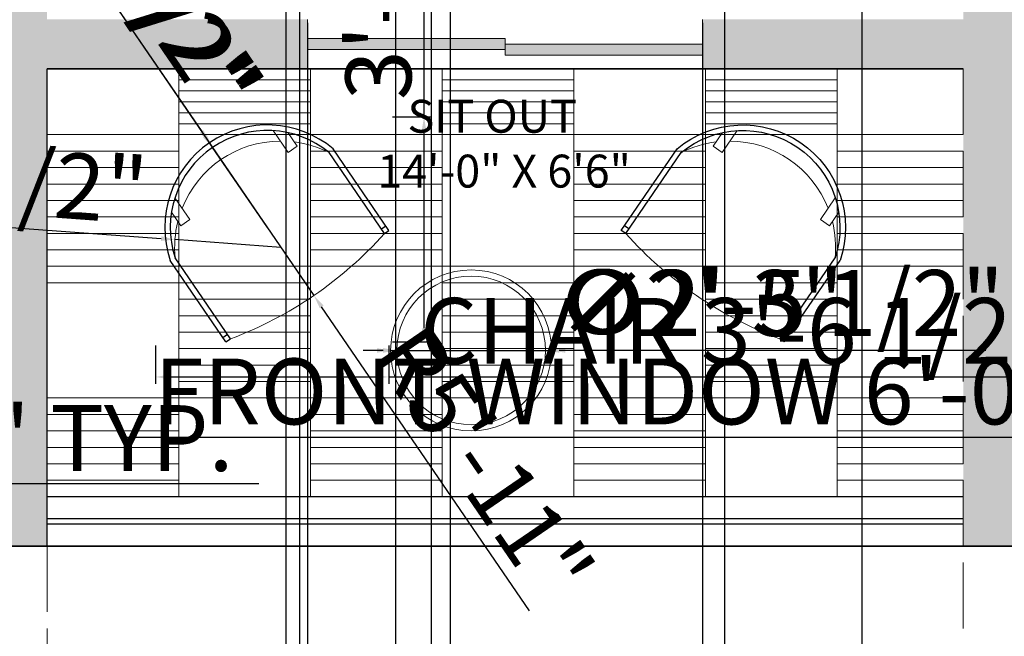
# Model space of a CAD drawing. Units: millimetres. Extents: x 542930 to 543750, y 628093 to 628738.
# Tile 5 of 14: x 543153 to 543333, y 628237 to 628350. Entities that reach past the tile are written whole.
import ezdxf

# ---------------------------------------------------------------- set-up
doc = ezdxf.new("R2010")
doc.units = ezdxf.units.MM
doc.linetypes.add('ACAD_ISO02W100', pattern=[15, 12, -3])
for name, color, linetype, lineweight in [('A-ANNO-DIMS', 2, 'Continuous', 18), ('A-FLOR-BELO', 4, 'ACAD_ISO02W100', 18), ('A-FLOR-EDGE', 9, 'Continuous', 25), ('A-FURN', 8, 'Continuous', 18), ('A-WALL', 7, 'Continuous', 35), ('DOORS', 30, 'Continuous', 18)]:
    doc.layers.add(name, color=color, linetype=linetype, lineweight=lineweight)
for name, color, linetype, lineweight, true_color in [('A-AREA-IDEN', 40, 'Continuous', 18, 0xf8d731), ('A-DOOR-PATT', 152, 'Continuous', 13, 0x2776bb), ('A-FLOR-DECK-PATT', 32, 'Continuous', 13, 0xcd6928), ('A-WALL-PATT', 251, 'Continuous', 13, 0x636466)]:
    doc.layers.add(name, color=color, linetype=linetype, lineweight=lineweight, true_color=true_color)
doc.layers.add('TEXT', color=220, linetype='Continuous')
doc.styles.get("Standard").update_dxf_attribs({"font": 'arial.ttf'})
doc.dimstyles.new('ISO-25', dxfattribs={"dimtxt": 12, "dimasz": 2.5, "dimexe": 1.25, "dimexo": 0.625, "dimtad": 1, "dimdec": 0, "dimlunit": 3, "dimtxsty": 'Standard', "dimcen": 2.5, "dimadec": 0, "dimazin": 0, "dimtfac": 1, "dimtdec": 0, "dimtmove": 0, "dimatfit": 3, "dimfxl": 1, "dimarcsym": 0})

# ---------------------------------------------------------------- blocks, each defined once
blk = doc.blocks.new('chair')
for p, q in [((543076.08, 628228.18), (543073.37, 628232.15)), ((543076.04, 628231.79), (543077.73, 628229.31)), ((543077.73, 628229.31), (543076.08, 628228.18)), ((543058.18, 628215.93), (543055.46, 628219.91)), ((543054.84, 628217.28), (543056.53, 628214.81)), ((543056.53, 628214.81), (543058.18, 628215.93))]:
    blk.add_line(p, q)
for centre, radius, start, end in [((543074.79, 628210.87), 19.38, 90.3414, 158.4163), ((543074.79, 628210.87), 19.38, 63.0526, 82.8533), ((543074.79, 628210.87), 19.38, 165.9044, 185.7051), ((543040.66, 628260.76), 71.07, 290.5394, 318.2183)]:
    blk.add_arc(centre, radius, start, end)
at = {"layer": 'TEXT'}
for p, q in [((543093.65, 628213.4), (543083.57, 628228.14)), ((543094.48, 628213.97), (543084.31, 628228.82)), ((543093.09, 628214.23), (543093.91, 628214.79)), ((543093.65, 628213.4), (543094.48, 628213.97)), ((543064.77, 628193.64), (543054.6, 628208.5)), ((543065.59, 628194.21), (543055.51, 628208.95)), ((543064.2, 628194.47), (543065.03, 628195.03)), ((543064.77, 628193.64), (543065.59, 628194.21))]:
    blk.add_line(p, q, dxfattribs=at)
for radius, start, end in [(18.7, 50.0638, 198.6939), (17.7, 50.5038, 198.2539)]:
    blk.add_arc((543072.31, 628214.49), radius, start, end, dxfattribs=at)
blk = doc.blocks.new('*D41')
at = {"layer": 'A-ANNO-DIMS', "color": 0, "lineweight": -2, "transparency": 16777216}
for p, q in [((543177.94, 628290.42), (543177.94, 628283.41)), ((543220.5, 628290.42), (543220.5, 628283.41)), ((543180.44, 628284.66), (543218, 628284.66)), ((543220.5, 628284.66), (543382.04, 628284.66))]:
    blk.add_line(p, q, dxfattribs=at)
at = {"layer": 'A-ANNO-DIMS', "color": 0, "transparency": 16777216}
for points in [[(543180.44, 628285.08), (543180.44, 628284.25), (543177.94, 628284.66)], [(543218, 628285.08), (543218, 628284.25), (543220.5, 628284.66)]]:
    blk.add_solid(points, dxfattribs=at)
at = {"layer": 'Defpoints', "color": 0, "transparency": 16777216}
for p in [(543177.94, 628291.05), (543220.5, 628291.05), (543220.5, 628284.66)]:
    blk.add_point(p, dxfattribs=at)
at = {"layer": 'A-ANNO-DIMS', "color": 0, "transparency": 16777216, "insert": (543302.52, 628291.5), "char_height": 12, "attachment_point": 5}
blk.add_mtext('CHAIR 3\'-6 1/2" TYP.', dxfattribs=at)
blk = doc.blocks.new('*D42')
at = {"layer": 'A-ANNO-DIMS', "color": 0, "lineweight": -2, "transparency": 16777216}
for p, q in [((543226.89, 628332.06), (543226.89, 628408.95)), ((543221.13, 628332.06), (543228.14, 628332.06)), ((543226.89, 628293.55), (543226.89, 628329.56)), ((543221.13, 628291.05), (543228.14, 628291.05))]:
    blk.add_line(p, q, dxfattribs=at)
at = {"layer": 'A-ANNO-DIMS', "color": 0, "transparency": 16777216}
for points in [[(543226.47, 628329.56), (543227.3, 628329.56), (543226.89, 628332.06)], [(543226.47, 628293.55), (543227.3, 628293.55), (543226.89, 628291.05)]]:
    blk.add_solid(points, dxfattribs=at)
at = {"layer": 'Defpoints', "color": 0, "transparency": 16777216}
for p in [(543220.5, 628332.06), (543226.89, 628332.06), (543220.5, 628291.05)]:
    blk.add_point(p, dxfattribs=at)
at = {"layer": 'A-ANNO-DIMS', "color": 0, "transparency": 16777216, "insert": (543220.13, 628371.75), "char_height": 12, "attachment_point": 5, "rotation": 90}
blk.add_mtext('3\'-5" TYP.', dxfattribs=at)
blk = doc.blocks.new('*D47')
at = {"layer": 'A-ANNO-DIMS', "color": 0, "lineweight": -2, "transparency": 16777216}
for p, q in [((542998.67, 628268.2), (542998.67, 628263.97)), ((543022.69, 628268.2), (543022.69, 628263.97)), ((543001.17, 628265.22), (543020.19, 628265.22)), ((543022.69, 628265.22), (543196.77, 628265.22))]:
    blk.add_line(p, q, dxfattribs=at)
at = {"layer": 'A-ANNO-DIMS', "color": 0, "transparency": 16777216}
for points in [[(543001.17, 628265.64), (543001.17, 628264.81), (542998.67, 628265.22)], [(543020.19, 628265.64), (543020.19, 628264.81), (543022.69, 628265.22)]]:
    blk.add_solid(points, dxfattribs=at)
at = {"layer": 'Defpoints', "color": 0, "transparency": 16777216}
for p in [(542998.67, 628268.83), (543022.69, 628268.83), (543022.69, 628265.22)]:
    blk.add_point(p, dxfattribs=at)
at = {"layer": 'A-ANNO-DIMS', "color": 0, "transparency": 16777216, "insert": (543110.98, 628271.97), "char_height": 12, "attachment_point": 5}
blk.add_mtext('END TABLE 2\'-0" TYP.', dxfattribs=at)
blk = doc.blocks.new('*D49')
at = {"layer": 'A-ANNO-DIMS', "color": 0, "lineweight": -2, "transparency": 16777216}
for p, q in [((543388.65, 628263.45), (543388.65, 628274.88)), ((543460.65, 628263.45), (543460.65, 628274.88)), ((543388.65, 628273.63), (543171.83, 628273.63)), ((543458.15, 628273.63), (543391.15, 628273.63))]:
    blk.add_line(p, q, dxfattribs=at)
at = {"layer": 'A-ANNO-DIMS', "color": 0, "transparency": 16777216}
for points in [[(543391.15, 628274.04), (543391.15, 628273.21), (543388.65, 628273.63)], [(543458.15, 628274.04), (543458.15, 628273.21), (543460.65, 628273.63)]]:
    blk.add_solid(points, dxfattribs=at)
at = {"layer": 'Defpoints', "color": 0, "transparency": 16777216}
for p in [(543388.65, 628273.63), (543388.65, 628262.83), (543460.65, 628262.83)]:
    blk.add_point(p, dxfattribs=at)
at = {"layer": 'A-ANNO-DIMS', "color": 0, "transparency": 16777216, "insert": (543278.99, 628280.46), "char_height": 12, "attachment_point": 5}
blk.add_mtext('FRONT WINDOW 6\'-0" TYP.', dxfattribs=at)
blk = doc.blocks.new('*D61')
at = {"layer": 'A-ANNO-DIMS', "color": 0, "lineweight": -2, "transparency": 16777216}
for p, q in [((543500.29, 628253.83), (543537.81, 628253.83)), ((543536.56, 628136.33), (543536.56, 628251.33)), ((543325.79, 628133.83), (543537.81, 628133.83))]:
    blk.add_line(p, q, dxfattribs=at)
at = {"layer": 'A-ANNO-DIMS', "color": 0, "transparency": 16777216}
for points in [[(543536.15, 628251.33), (543536.98, 628251.33), (543536.56, 628253.83)], [(543536.15, 628136.33), (543536.98, 628136.33), (543536.56, 628133.83)]]:
    blk.add_solid(points, dxfattribs=at)
at = {"layer": 'Defpoints', "color": 0, "transparency": 16777216}
for p in [(543499.67, 628253.83), (543536.56, 628253.83), (543325.17, 628133.83)]:
    blk.add_point(p, dxfattribs=at)
at = {"layer": 'A-ANNO-DIMS', "color": 0, "transparency": 16777216, "insert": (543529.81, 628193.83), "char_height": 12, "attachment_point": 5, "rotation": 90}
blk.add_mtext('10\'-0"', dxfattribs=at)
blk = doc.blocks.new('*D71')
at = {"layer": 'A-ANNO-DIMS', "color": 0, "lineweight": -2, "transparency": 16777216}
for p, q in [((543201.67, 628544.2), (543201.67, 628103.84)), ((543281.67, 628544.2), (543281.67, 628103.84)), ((543204.17, 628105.09), (543279.17, 628105.09))]:
    blk.add_line(p, q, dxfattribs=at)
at = {"layer": 'A-ANNO-DIMS', "color": 0, "transparency": 16777216}
for points in [[(543204.17, 628105.5), (543204.17, 628104.67), (543201.67, 628105.09)], [(543279.17, 628105.5), (543279.17, 628104.67), (543281.67, 628105.09)]]:
    blk.add_solid(points, dxfattribs=at)
at = {"layer": 'Defpoints', "color": 0, "transparency": 16777216}
for p in [(543201.67, 628544.83), (543281.67, 628544.83), (543281.67, 628105.09)]:
    blk.add_point(p, dxfattribs=at)
at = {"layer": 'A-ANNO-DIMS', "color": 0, "transparency": 16777216, "insert": (543241.67, 628111.84), "char_height": 12, "attachment_point": 5}
blk.add_mtext('6\'-8"', dxfattribs=at)
blk = doc.blocks.new('*D76')
at = {"layer": 'A-ANNO-DIMS', "color": 0, "lineweight": -2, "transparency": 16777216}
for p, q in [((543205.67, 628349.2), (543205.67, 628103.84)), ((543277.67, 628349.2), (543277.67, 628103.84)), ((543208.17, 628105.09), (543275.17, 628105.09))]:
    blk.add_line(p, q, dxfattribs=at)
at = {"layer": 'A-ANNO-DIMS', "color": 0, "transparency": 16777216}
for points in [[(543208.17, 628105.5), (543208.17, 628104.67), (543205.67, 628105.09)], [(543275.17, 628105.5), (543275.17, 628104.67), (543277.67, 628105.09)]]:
    blk.add_solid(points, dxfattribs=at)
at = {"layer": 'Defpoints', "color": 0, "transparency": 16777216}
for p in [(543205.67, 628349.83), (543277.67, 628349.83), (543277.67, 628105.09)]:
    blk.add_point(p, dxfattribs=at)
at = {"layer": 'A-ANNO-DIMS', "color": 0, "transparency": 16777216, "insert": (543241.67, 628111.84), "char_height": 12, "attachment_point": 5}
blk.add_mtext('6\'-0"', dxfattribs=at)
blk = doc.blocks.new('*D79')
at = {"layer": 'A-ANNO-DIMS', "color": 0, "lineweight": -2, "transparency": 16777216}
for p, q in [((543204.19, 628433.96), (543204.19, 628103.84)), ((543228.16, 628433.96), (543228.16, 628103.84)), ((543206.69, 628105.09), (543225.66, 628105.09)), ((543228.16, 628105.09), (543264.02, 628105.09))]:
    blk.add_line(p, q, dxfattribs=at)
at = {"layer": 'A-ANNO-DIMS', "color": 0, "transparency": 16777216}
for points in [[(543206.69, 628105.5), (543206.69, 628104.67), (543204.19, 628105.09)], [(543225.66, 628105.5), (543225.66, 628104.67), (543228.16, 628105.09)]]:
    blk.add_solid(points, dxfattribs=at)
at = {"layer": 'Defpoints', "color": 0, "transparency": 16777216}
for p in [(543204.19, 628434.59), (543228.16, 628434.59), (543228.16, 628105.09)]:
    blk.add_point(p, dxfattribs=at)
at = {"layer": 'A-ANNO-DIMS', "color": 0, "transparency": 16777216, "insert": (543247.34, 628111.84), "char_height": 12, "attachment_point": 5}
blk.add_mtext('2\'-0"', dxfattribs=at)
blk = doc.blocks.new('*D81')
at = {"layer": 'A-ANNO-DIMS', "color": 0, "lineweight": -2, "transparency": 16777216}
for p, q in [((543228.16, 628433.96), (543228.16, 628103.84)), ((543306.67, 628434.2), (543306.67, 628103.84)), ((543230.66, 628105.09), (543304.17, 628105.09))]:
    blk.add_line(p, q, dxfattribs=at)
at = {"layer": 'A-ANNO-DIMS', "color": 0, "transparency": 16777216}
for points in [[(543230.66, 628105.5), (543230.66, 628104.67), (543228.16, 628105.09)], [(543304.17, 628105.5), (543304.17, 628104.67), (543306.67, 628105.09)]]:
    blk.add_solid(points, dxfattribs=at)
at = {"layer": 'Defpoints', "color": 0, "transparency": 16777216}
for p in [(543228.16, 628434.59), (543306.67, 628434.83), (543306.67, 628105.09)]:
    blk.add_point(p, dxfattribs=at)
at = {"layer": 'A-ANNO-DIMS', "color": 0, "transparency": 16777216, "insert": (543267.41, 628111.92), "char_height": 12, "attachment_point": 5}
blk.add_mtext('6\'-6 1/2"', dxfattribs=at)
blk = doc.blocks.new('*D87')
at = {"layer": 'A-ANNO-DIMS', "color": 0, "lineweight": -2, "transparency": 16777216}
for p, q in [((543221.67, 628580.2), (543221.67, 628103.84)), ((543231.67, 628580.2), (543231.67, 628103.84)), ((543224.17, 628105.09), (543229.17, 628105.09)), ((543231.67, 628105.09), (543276.64, 628105.09))]:
    blk.add_line(p, q, dxfattribs=at)
at = {"layer": 'A-ANNO-DIMS', "color": 0, "transparency": 16777216}
for points in [[(543224.17, 628105.5), (543224.17, 628104.67), (543221.67, 628105.09)], [(543229.17, 628105.5), (543229.17, 628104.67), (543231.67, 628105.09)]]:
    blk.add_solid(points, dxfattribs=at)
at = {"layer": 'Defpoints', "color": 0, "transparency": 16777216}
for p in [(543221.67, 628580.83), (543231.67, 628580.83), (543231.67, 628105.09)]:
    blk.add_point(p, dxfattribs=at)
at = {"layer": 'A-ANNO-DIMS', "color": 0, "transparency": 16777216, "insert": (543255.4, 628111.84), "char_height": 12, "attachment_point": 5}
blk.add_mtext('0\'-10"', dxfattribs=at)
blk = doc.blocks.new('*D88')
at = {"layer": 'A-ANNO-DIMS', "color": 0, "lineweight": -2, "transparency": 16777216}
for p, q in [((543218.3, 628289.5), (543215.8, 628289.5)), ((543220.8, 628289.5), (543250.15, 628289.5)), ((543329.31, 628289.5), (543252.65, 628289.5))]:
    blk.add_line(p, q, dxfattribs=at)
at = {"layer": 'A-ANNO-DIMS', "color": 0, "transparency": 16777216}
for points in [[(543218.3, 628289.91), (543218.3, 628289.08), (543220.8, 628289.5)], [(543252.65, 628289.91), (543252.65, 628289.08), (543250.15, 628289.5)]]:
    blk.add_solid(points, dxfattribs=at)
at = {"layer": 'Defpoints', "color": 0, "transparency": 16777216}
for p in [(543220.8, 628289.5), (543250.15, 628289.5)]:
    blk.add_point(p, dxfattribs=at)
at = {"layer": 'A-ANNO-DIMS', "color": 0, "transparency": 16777216, "insert": (543292.23, 628296.59), "char_height": 12, "attachment_point": 5, "rotation": 0.0001}
blk.add_mtext('∅2\'-5 1/2"', dxfattribs=at)
blk = doc.blocks.new('*D89')
at = {"layer": 'A-ANNO-DIMS', "color": 0, "lineweight": -2, "transparency": 16777216}
for p, q in [((543219.43, 628289.5), (543216.93, 628289.5)), ((543221.93, 628289.5), (543249.02, 628289.5)), ((543300.22, 628289.5), (543251.52, 628289.5))]:
    blk.add_line(p, q, dxfattribs=at)
at = {"layer": 'A-ANNO-DIMS', "color": 0, "transparency": 16777216}
for points in [[(543219.43, 628289.91), (543219.43, 628289.08), (543221.93, 628289.5)], [(543251.52, 628289.91), (543251.52, 628289.08), (543249.02, 628289.5)]]:
    blk.add_solid(points, dxfattribs=at)
at = {"layer": 'Defpoints', "color": 0, "transparency": 16777216}
for p in [(543221.93, 628289.5), (543249.02, 628289.5)]:
    blk.add_point(p, dxfattribs=at)
at = {"layer": 'A-ANNO-DIMS', "color": 0, "transparency": 16777216, "insert": (543277.12, 628296.59), "char_height": 12, "attachment_point": 5, "rotation": 0.0001}
blk.add_mtext('∅2\'-3"', dxfattribs=at)
blk = doc.blocks.new('*D92')
at = {"layer": 'A-ANNO-DIMS', "color": 0, "lineweight": -2, "transparency": 16777216}
for p, q in [((543166.68, 628358.16), (543206.81, 628299.51)), ((543246.12, 628242.05), (543208.22, 628297.45))]:
    blk.add_line(p, q, dxfattribs=at)
at = {"layer": 'A-ANNO-DIMS', "color": 0, "transparency": 16777216}
blk.add_solid([(543208.57, 628297.68), (543207.88, 628297.21), (543206.81, 628299.51)], dxfattribs=at)
at = {"layer": 'Defpoints', "color": 0, "transparency": 16777216}
for p in [(543166.68, 628358.16), (543206.81, 628299.51)]:
    blk.add_point(p, dxfattribs=at)
at = {"layer": 'A-ANNO-DIMS', "color": 0, "transparency": 16777216, "insert": (543236.46, 628268.13), "char_height": 12, "attachment_point": 5, "rotation": 304.379}
blk.add_mtext('R5\'-11"', dxfattribs=at)
blk = doc.blocks.new('*D93')
at = {"layer": 'A-ANNO-DIMS', "color": 0, "lineweight": -2, "transparency": 16777216}
for p, q in [((543078.39, 628317.26), (543178.99, 628309.88)), ((543200.81, 628308.28), (543181.49, 628309.7))]:
    blk.add_line(p, q, dxfattribs=at)
at = {"layer": 'A-ANNO-DIMS', "color": 0, "transparency": 16777216}
blk.add_solid([(543179.02, 628310.3), (543178.96, 628309.46), (543181.49, 628309.7)], dxfattribs=at)
at = {"layer": 'Defpoints', "color": 0, "transparency": 16777216}
for p in [(543181.49, 628309.7), (543200.81, 628308.28)]:
    blk.add_point(p, dxfattribs=at)
at = {"layer": 'A-ANNO-DIMS', "color": 0, "transparency": 16777216, "insert": (543127.94, 628320.48), "char_height": 12, "attachment_point": 5, "rotation": 355.8053}
blk.add_mtext('3X R1\'-7 1/2"', dxfattribs=at)
blk = doc.blocks.new('*D94')
at = {"layer": 'A-ANNO-DIMS', "color": 0, "lineweight": -2, "transparency": 16777216}
for p, q in [((543143.96, 628391.37), (543186.37, 628329.39)), ((543198.34, 628311.9), (543187.78, 628327.33))]:
    blk.add_line(p, q, dxfattribs=at)
at = {"layer": 'A-ANNO-DIMS', "color": 0, "transparency": 16777216}
blk.add_solid([(543186.71, 628329.63), (543186.02, 628329.15), (543187.78, 628327.33)], dxfattribs=at)
at = {"layer": 'Defpoints', "color": 0, "transparency": 16777216}
for p in [(543187.78, 628327.33), (543198.34, 628311.9)]:
    blk.add_point(p, dxfattribs=at)
at = {"layer": 'A-ANNO-DIMS', "color": 0, "transparency": 16777216, "insert": (543170.1, 628365.27), "char_height": 12, "attachment_point": 5, "rotation": 304.3793}
blk.add_mtext('R1\'-6 1/2"', dxfattribs=at)
blk = doc.blocks.new('*D95')
at = {"layer": 'A-ANNO-DIMS', "color": 0, "lineweight": -2, "transparency": 16777216}
for p, q in [((543144.53, 628390.54), (543186.93, 628328.57)), ((543198.34, 628311.9), (543188.34, 628326.5))]:
    blk.add_line(p, q, dxfattribs=at)
at = {"layer": 'A-ANNO-DIMS', "color": 0, "transparency": 16777216}
blk.add_solid([(543187.28, 628328.8), (543186.59, 628328.33), (543188.34, 628326.5)], dxfattribs=at)
at = {"layer": 'Defpoints', "color": 0, "transparency": 16777216}
for p in [(543188.34, 628326.5), (543198.34, 628311.9)]:
    blk.add_point(p, dxfattribs=at)
at = {"layer": 'A-ANNO-DIMS', "color": 0, "transparency": 16777216, "insert": (543170.66, 628364.44), "char_height": 12, "attachment_point": 5, "rotation": 304.3778}
blk.add_mtext('R1\'-5 1/2"', dxfattribs=at)

msp = doc.modelspace()

# ---------------------------------------------------------------- hatches: boundary and pattern name
at = {"layer": 'A-DOOR-PATT'}
h = msp.add_hatch(color=256, dxfattribs=at)
h.dxf.hatch_style = 1
h.paths.add_polyline_path([(543241.67, 628346.33), (543205.67, 628346.33), (543205.67, 628344.33), (543241.67, 628344.33)])
h = msp.add_hatch(color=256, dxfattribs=at)
h.dxf.hatch_style = 1
h.paths.add_polyline_path([(543277.67, 628345.33), (543241.67, 628345.33), (543241.67, 628344.33), (543241.67, 628343.33), (543277.67, 628343.33)])
at = {"layer": 'A-FLOR-DECK-PATT'}
h = msp.add_hatch(dxfattribs=at)
h.set_pattern_fill('LINE', color=256, scale=0.629922088, style=0)
h.paths.add_polyline_path([(543182.17, 628328.88), (543206.17, 628328.88), (543206.17, 628340.77), (543182.17, 628340.77)])
h = msp.add_hatch(dxfattribs=at)
h.set_pattern_fill('LINE', color=256, scale=0.629922088, style=0)
h.paths.add_polyline_path([(543230.17, 628328.88), (543254.17, 628328.88), (543254.17, 628340.77), (543230.17, 628340.77)])
h = msp.add_hatch(dxfattribs=at)
h.set_pattern_fill('LINE', color=256, scale=0.629922088, style=0)
h.paths.add_polyline_path([(543278.17, 628328.88), (543302.17, 628328.88), (543302.17, 628340.77), (543278.17, 628340.77)])
h = msp.add_hatch(dxfattribs=at)
h.set_pattern_fill('LINE', color=256, scale=0.94488163, style=0)
h.paths.add_polyline_path([(543158.17, 628304.88), (543182.17, 628304.88), (543182.17, 628328.77), (543158.17, 628328.77)])
h = msp.add_hatch(dxfattribs=at)
h.set_pattern_fill('LINE', color=256, scale=0.94488163, style=0)
h.paths.add_polyline_path([(543206.17, 628304.88), (543230.17, 628304.88), (543230.17, 628328.77), (543206.17, 628328.77)])
h = msp.add_hatch(dxfattribs=at)
h.set_pattern_fill('LINE', color=256, scale=0.94488163, style=0)
h.paths.add_polyline_path([(543254.17, 628304.88), (543278.17, 628304.88), (543278.17, 628328.77), (543254.17, 628328.77)])
h = msp.add_hatch(dxfattribs=at)
h.set_pattern_fill('LINE', color=256, scale=0.94488163, style=0)
h.paths.add_polyline_path([(543302.17, 628304.88), (543325.17, 628304.88), (543325.17, 628328.77), (543302.17, 628328.77)])
h = msp.add_hatch(dxfattribs=at)
h.set_pattern_fill('LINE', color=256, scale=0.94488163, style=0)
h.paths.add_polyline_path([(543230.17, 628280.88), (543254.17, 628280.88), (543254.17, 628304.77), (543230.17, 628304.77)])
h = msp.add_hatch(dxfattribs=at)
h.set_pattern_fill('LINE', color=256, scale=0.94488163, style=0)
h.paths.add_polyline_path([(543278.17, 628280.88), (543302.17, 628280.88), (543302.17, 628304.77), (543278.17, 628304.77)])
h = msp.add_hatch(dxfattribs=at)
h.set_pattern_fill('LINE', color=256, scale=0.94488163, style=0)
h.paths.add_polyline_path([(543182.17, 628280.88), (543206.17, 628280.88), (543206.17, 628301.77), (543182.17, 628301.77)])
h = msp.add_hatch(dxfattribs=at)
h.set_pattern_fill('LINE', color=256, scale=0.94488163, style=0)
h.paths.add_polyline_path([(543158.17, 628262.88), (543182.17, 628262.88), (543182.17, 628280.77), (543158.17, 628280.77)])
h = msp.add_hatch(dxfattribs=at)
h.set_pattern_fill('LINE', color=256, scale=0.94488163, style=0)
h.paths.add_polyline_path([(543206.17, 628262.88), (543230.17, 628262.88), (543230.17, 628280.77), (543206.17, 628280.77)])
h = msp.add_hatch(dxfattribs=at)
h.set_pattern_fill('LINE', color=256, scale=0.94488163, style=0)
h.paths.add_polyline_path([(543254.17, 628262.88), (543278.17, 628262.88), (543278.17, 628280.77), (543254.17, 628280.77)])
h = msp.add_hatch(dxfattribs=at)
h.set_pattern_fill('LINE', color=256, scale=0.94488163, style=0)
h.paths.add_polyline_path([(543302.17, 628262.88), (543325.17, 628262.88), (543325.17, 628280.77), (543302.17, 628280.77)])
at = {"layer": 'A-WALL-PATT'}
h = msp.add_hatch(color=256, dxfattribs=at)
h.dxf.hatch_style = 1
h.paths.add_polyline_path([(543388.65, 628262.83), (543374.28, 628262.83), (543334.17, 628262.83), (543334.17, 628439.36), (543325.17, 628439.36), (543325.17, 628349.83), (543277.67, 628349.83), (543277.67, 628340.83), (543325.17, 628340.83), (543325.17, 628253.83), (543388.65, 628253.83)])
h = msp.add_hatch(color=256, dxfattribs=at)
h.dxf.hatch_style = 1
h.paths.add_polyline_path([(543158.17, 628340.83), (543205.67, 628340.83), (543205.67, 628349.83), (543158.17, 628349.83), (543158.17, 628360.23), (543149.17, 628360.23), (543149.17, 628262.83), (543094.69, 628262.83), (543094.69, 628253.83), (543158.17, 628253.83)])

# ---------------------------------------------------------------- linework, layer by layer
at = {"layer": 'A-FLOR-BELO'}
for p, q in [((543325.17, 628340.83), (543325.17, 628133.83)), ((543158.17, 628253.83), (543158.17, 628133.79))]:
    msp.add_line(p, q, dxfattribs=at)
at = {"layer": 'A-FLOR-DECK-PATT'}
for p, q in [((543182.17, 628262.83), (543182.17, 628340.83)), ((543206.17, 628262.83), (543206.17, 628340.83)), ((543230.17, 628262.83), (543230.17, 628340.83)), ((543254.17, 628262.83), (543254.17, 628340.83)), ((543278.17, 628262.83), (543278.17, 628340.83)), ((543302.17, 628262.83), (543302.17, 628340.83)), ((543325.17, 628328.83), (543158.17, 628328.83)), ((543325.17, 628304.83), (543158.17, 628304.83)), ((543206.17, 628301.83), (543158.17, 628301.83)), ((543325.17, 628280.83), (543158.17, 628280.83))]:
    msp.add_line(p, q, dxfattribs=at)
at = {"layer": 'A-FLOR-EDGE'}
for p, q in [((543158.17, 628253.83), (543158.17, 628340.83)), ((543325.17, 628262.83), (543158.17, 628262.83)), ((543325.17, 628258.83), (543158.17, 628258.83))]:
    msp.add_line(p, q, dxfattribs=at)
msp.add_lwpolyline([(543325.17, 628257.83), (543158.17, 628257.83)], dxfattribs=at)
at = {"layer": 'A-FURN'}
for radius in [14.67, 13.54]:
    msp.add_circle((543235.47, 628289.5), radius, dxfattribs=at)
at = {"layer": 'A-WALL'}
msp.add_line((543325.17, 628340.83), (543158.17, 628340.83), dxfattribs=at)
msp.add_lwpolyline([(543499.67, 628253.83), (542983.67, 628253.83), (542983.67, 628589.83)], dxfattribs=at)
at = {"layer": 'DOORS'}
for p, q in [((543205.67, 628349.83), (543205.67, 628340.83)), ((543277.67, 628349.83), (543277.67, 628340.83)), ((543205.67, 628346.33), (543241.67, 628346.33)), ((543241.67, 628346.33), (543241.67, 628343.33)), ((543205.67, 628344.33), (543241.67, 628344.33)), ((543241.67, 628345.33), (543277.67, 628345.33)), ((543241.67, 628343.33), (543277.67, 628343.33))]:
    msp.add_line(p, q, dxfattribs=at)

# ---------------------------------------------------------------- block references
at = {"layer": 'A-FURN'}
msp.add_blockref('chair', (126.02, 97.41), dxfattribs=at)
at = {"layer": 'A-FURN', "xscale": -1}
msp.add_blockref('chair', (1086357.31, 97.41), dxfattribs=at)

# ---------------------------------------------------------------- texts
at = {"layer": 'A-AREA-IDEN', "insert": (543216.54, 628335.18), "char_height": 6, "attachment_point": 1}
msp.add_mtext_dynamic_manual_height_columns('    SIT OUT\\P 14\'-0" X 6\'6"', width=77.2525, gutter_width=12.5, heights=[0], dxfattribs=at)

# ---------------------------------------------------------------- dimensions: what is measured, and where the dimension line sits
at = {"layer": 'A-ANNO-DIMS'}
for base, p1, p2, picture, middle in [((543231.67, 628105.09), (543221.67, 628580.83), (543231.67, 628580.83), '*D87', (543255.4, 628111.84)), ((543281.67, 628105.09), (543201.67, 628544.83), (543281.67, 628544.83), '*D71', (543241.67, 628111.84)), ((543228.16, 628105.09), (543204.19, 628434.59), (543228.16, 628434.59), '*D79', (543247.34, 628111.84)), ((543306.67, 628105.09), (543228.16, 628434.59), (543306.67, 628434.83), '*D81', (543267.41, 628111.92)), ((543277.67, 628105.09), (543205.67, 628349.83), (543277.67, 628349.83), '*D76', (543241.67, 628111.84))]:
    dim = msp.add_linear_dim(base=base, p1=p1, p2=p2, dimstyle='ISO-25', override={"dimdec": 1, "dimlfac": 1, "dimrnd": 0, "dimzin": 1, "dimdsep": 46, "dimlunit": 4, "dimfrac": 2}, dxfattribs=at)
    dim.commit()
    dim.dimension.update_dxf_attribs({"geometry": picture, "text_midpoint": middle})
for base, p1, p2, angle, text, picture, middle in [((543226.89, 628332.06), (543220.5, 628291.05), (543220.5, 628332.06), 90, '<> TYP.', '*D42', (543220.13, 628371.75)), ((543388.65, 628273.63), (543460.65, 628262.83), (543388.65, 628262.83), 180, 'FRONT WINDOW <> TYP.', '*D49', (543278.99, 628280.46))]:
    dim = msp.add_linear_dim(base=base, p1=p1, p2=p2, angle=angle, text=text, dimstyle='ISO-25', override={"dimdec": 1, "dimlfac": 1, "dimrnd": 0, "dimzin": 1, "dimdsep": 46, "dimlunit": 4, "dimfrac": 2}, dxfattribs=at)
    dim.commit()
    dim.dimension.update_dxf_attribs({"geometry": picture, "text_midpoint": middle})
for mpoint, picture, middle in [((543187.78, 628327.33), '*D94', (543170.1, 628365.27)), ((543188.34, 628326.5), '*D95', (543170.66, 628364.44))]:
    dim = msp.add_radius_dim(center=(543198.34, 628311.9), mpoint=mpoint, dimstyle='ISO-25', override={"dimdec": 1, "dimlfac": 1, "dimrnd": 0, "dimzin": 1, "dimdsep": 46, "dimlunit": 4, "dimfrac": 2}, dxfattribs=at)
    dim.commit()
    dim.dimension.update_dxf_attribs({"geometry": picture, "text_midpoint": middle})
dim = msp.add_radius_dim(center=(543166.68, 628358.16), mpoint=(543206.81, 628299.51), dimstyle='ISO-25', override={"dimdec": 1, "dimlfac": 1, "dimrnd": 0, "dimzin": 1, "dimdsep": 46, "dimlunit": 4, "dimfrac": 2}, dxfattribs=at)
dim.commit()
dim.dimension.update_dxf_attribs({"geometry": '*D92', "text_midpoint": (543230.89, 628264.32), "dimtype": 164})
dim = msp.add_radius_dim(center=(543200.81, 628308.28), mpoint=(543181.49, 628309.7), text='3X <>', dimstyle='ISO-25', override={"dimdec": 1, "dimlfac": 1, "dimrnd": 0, "dimzin": 1, "dimdsep": 46, "dimlunit": 4, "dimfrac": 2}, dxfattribs=at)
dim.commit()
dim.dimension.update_dxf_attribs({"geometry": '*D93', "text_midpoint": (543127.94, 628320.48)})
for base, p1, p2, text, picture, middle in [((543220.5, 628284.66), (543177.94, 628291.05), (543220.5, 628291.05), 'CHAIR <> TYP.', '*D41', (543302.52, 628291.5)), ((543022.69, 628265.22), (542998.67, 628268.83), (543022.69, 628268.83), 'END TABLE <> TYP.', '*D47', (543110.98, 628271.97))]:
    dim = msp.add_linear_dim(base=base, p1=p1, p2=p2, text=text, dimstyle='ISO-25', override={"dimdec": 1, "dimlfac": 1, "dimrnd": 0, "dimzin": 1, "dimdsep": 46, "dimlunit": 4, "dimfrac": 2}, dxfattribs=at)
    dim.commit()
    dim.dimension.update_dxf_attribs({"geometry": picture, "text_midpoint": middle})
for p1, p2, picture, middle in [((543220.8009, 628289.4979), (543250.1451, 628289.498), '*D88', (543292.2285, 628289.4981)), ((543221.93, 628289.5), (543249.02, 628289.5), '*D89', (543277.12, 628289.5))]:
    dim = msp.add_diameter_dim_2p(p1=p1, p2=p2, dimstyle='ISO-25', override={"dimdec": 1, "dimlfac": 1, "dimrnd": 0, "dimzin": 1, "dimdsep": 46, "dimlunit": 4, "dimfrac": 2}, dxfattribs=at)
    dim.commit()
    dim.dimension.update_dxf_attribs({"geometry": picture, "text_midpoint": middle})
dim = msp.add_linear_dim(base=(543536.56, 628253.83), p1=(543325.17, 628133.83), p2=(543499.67, 628253.83), angle=90, dimstyle='ISO-25', override={"dimdec": 1, "dimlfac": 1, "dimrnd": 0, "dimzin": 1, "dimdsep": 46, "dimlunit": 4, "dimfrac": 2}, dxfattribs=at)
dim.commit()
dim.dimension.update_dxf_attribs({"geometry": '*D61', "text_midpoint": (543529.81, 628193.83)})

doc.saveas('drawing.dxf')
